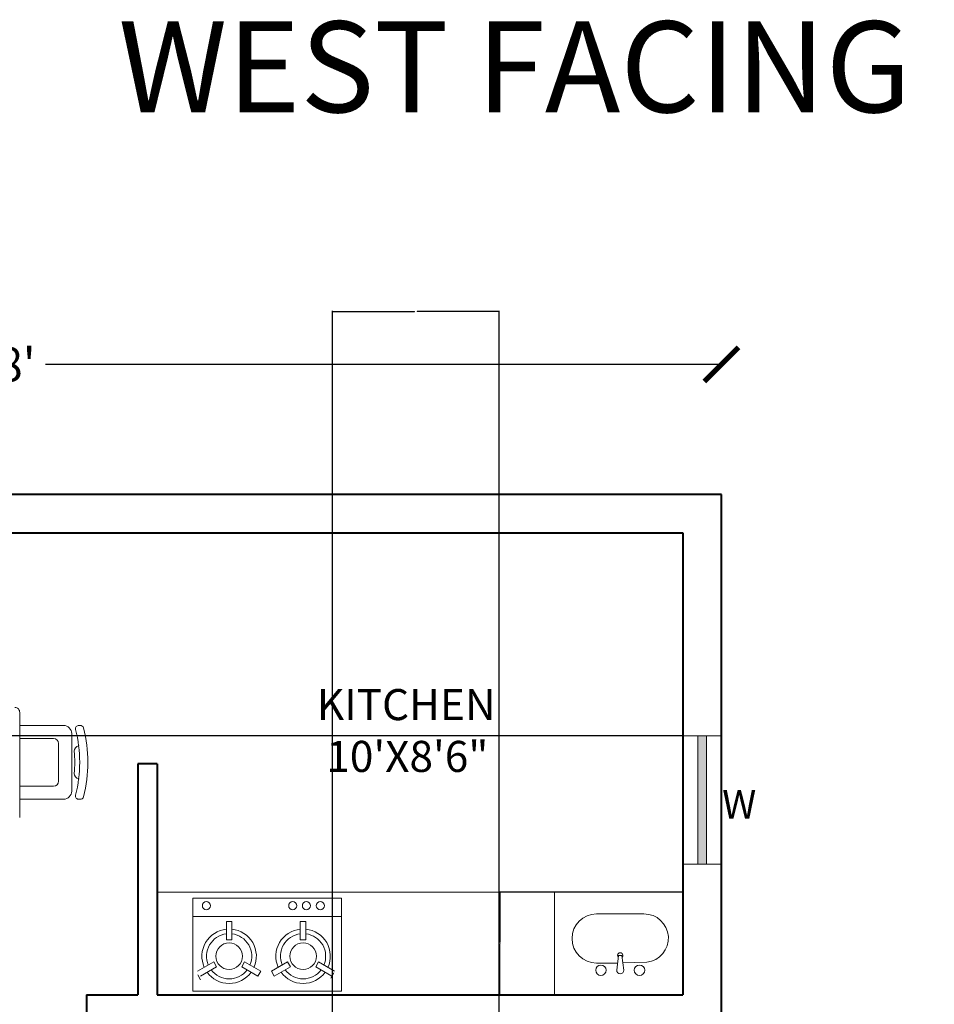
# Model space of a CAD drawing. Units: inches. Extents: x 182 to 1022, y -617 to 111.
# Tile 22 of 33: x 401 to 615, y -120 to 111. Entities that reach past the tile are written whole.
import ezdxf

# ---------------------------------------------------------------- set-up
doc = ezdxf.new("R2010")
doc.units = ezdxf.units.IN
doc.header["$MEASUREMENT"] = 0
for name, color, linetype, lineweight in [('A-ANNO-DIMS', 2, 'Continuous', 18), ('A-ANNO-IDEN', 1, 'Continuous', 18), ('A-ANNO-TEXT', 8, 'Continuous', 20), ('A-AREA-IDEN', 8, 'Continuous', 18), ('A-EQPM', 50, 'Continuous', 18), ('A-FLOR-CASE', 1, 'Continuous', 20), ('A-FLOR-FIXT', 50, 'Continuous', 18), ('A-GLAZ-PATT', 5, 'Continuous', 13), ('wall', 1, 'Continuous', 40), ('wind', 5, 'Continuous', 20)]:
    doc.layers.add(name, color=color, linetype=linetype, lineweight=lineweight)
doc.layers.add('furniture', color=50, linetype='Continuous', lineweight=15, transparency=0.8)
doc.styles.get("Standard").update_dxf_attribs({"font": 'arial.ttf'})
doc.dimstyles.get("Standard").update_dxf_attribs({"dimtxt": 0.18, "dimasz": 0.18, "dimexe": 0.18, "dimexo": 0.0625, "dimgap": 0.09, "dimtad": 0, "dimtih": 1, "dimtoh": 1, "dimdec": 1, "dimzin": 0, "dimdsep": 46, "dimlunit": 4, "dimtxsty": 'Standard', "dimcen": 0.09, "dimadec": 0, "dimazin": 0, "dimtfac": 1, "dimtdec": 1, "dimtofl": 0, "dimtmove": 0, "dimatfit": 3, "dimfxl": 1, "dimtolj": 1, "dimtzin": 0, "dimarcsym": 0})

# ---------------------------------------------------------------- blocks, each defined once
blk = doc.blocks.new('_ArchTick')
at = {"color": 0, "linetype": 'ByBlock', "const_width": 0.15}
blk.add_lwpolyline([(-0.5, -0.5), (0.5, 0.5)], dxfattribs=at)
blk = doc.blocks.new('*D5')
at = {"layer": 'A-ANNO-DIMS', "color": 0, "lineweight": -2, "transparency": 16777216}
for p, q in [((229.36, 30.06), (387.5, 30.06)), ((565.36, 30.06), (407.22, 30.06))]:
    blk.add_line(p, q, dxfattribs=at)
at = {"layer": 'Defpoints', "color": 0, "transparency": 16777216}
for p in [(565.36, 30.06), (229.36, -0.37), (565.36, -0.37)]:
    blk.add_point(p, dxfattribs=at)
at = {"layer": 'A-ANNO-DIMS', "color": 0, "lineweight": -2, "transparency": 16777216, "xscale": 8, "yscale": 8, "zscale": 8, "rotation": 180}
blk.add_blockref('_ArchTick', (229.36, 30.06), dxfattribs=at)
at = {"layer": 'A-ANNO-DIMS', "color": 0, "lineweight": -2, "transparency": 16777216, "xscale": 8, "yscale": 8, "zscale": 8}
blk.add_blockref('_ArchTick', (565.36, 30.06), dxfattribs=at)
at = {"layer": 'A-ANNO-DIMS', "color": 0, "transparency": 16777216, "insert": (397.36, 30.06), "char_height": 8, "attachment_point": 5}
blk.add_mtext("\\A1;28'", dxfattribs=at)
blk = doc.blocks.new('DINING-CHAIR-END')
for p, q in [((5.53, 17.27), (5.92, 17.27)), ((5.7, 17.27), (15.95, 17.27)), ((3.78, 1.92), (3.78, 15.35)), ((8.01, 14.2), (15.95, 14.2)), ((2.16, 12.47), (2.04, 12.47)), ((6.85, 4.22), (6.85, 13.05)), ((2.16, 4.8), (2.04, 4.8)), ((15.95, 3.07), (8.01, 3.07)), ((5.92, 0), (5.53, 0)), ((15.95, 0), (5.7, 0))]:
    blk.add_line(p, q)
for centre, radius, start, end in [((32.95, 8.63), 32.96, 165.853, 194.147), ((1.74, 16.5), 0.768, 84.0784, 165.853), ((1.94, 18.41), 1.15, 264.0784, 275.9216), ((32.95, 8.63), 31.04, 165.6786, 194.3214), ((2.14, 16.5), 0.768, 345.6786, 95.9216), ((5.7, 15.35), 1.92, 90, 180), ((8.01, 13.05), 1.15, 90, 180), ((2.04, 11.32), 1.15, 355.0346, 83.9719), ((32.95, 8.63), 29.89, 175.0346, 184.9654), ((2.04, 5.95), 1.15, 276.0281, 4.9654), ((8.01, 4.22), 1.15, 180, 270), ((1.74, 0.77), 0.768, 194.147, 275.9216), ((1.94, -1.14), 1.15, 84.0784, 95.9216), ((2.14, 0.77), 0.768, 264.0784, 14.3214), ((5.7, 1.92), 1.92, 180, 270)]:
    blk.add_arc(centre, radius, start, end)
blk = doc.blocks.new('*D43')
at = {"layer": 'A-ANNO-DIMS', "color": 0, "lineweight": -2, "transparency": 16777216}
for p, q in [((556.3, -9.37), (186.38, -9.37)), ((186.56, -9.55), (186.56, -32.91)), ((186.56, -56.63), (186.56, -33.28)), ((556.3, -56.81), (186.38, -56.81))]:
    blk.add_line(p, q, dxfattribs=at)
at = {"layer": 'A-ANNO-DIMS', "color": 0, "transparency": 16777216}
for points in [[(186.53, -9.55), (186.59, -9.55), (186.56, -9.37)], [(186.53, -56.63), (186.59, -56.63), (186.56, -56.81)]]:
    blk.add_solid(points, dxfattribs=at)
at = {"layer": 'Defpoints', "color": 0, "transparency": 16777216}
for p in [(556.36, -9.37), (186.56, -56.81), (556.36, -56.81)]:
    blk.add_point(p, dxfattribs=at)
at = {"layer": 'A-ANNO-DIMS', "color": 0, "transparency": 16777216, "insert": (186.56, -33.09), "char_height": 0.18, "attachment_point": 5}
blk.add_mtext('\\A1;3\'-11 1/2"', dxfattribs=at)
blk = doc.blocks.new('*D44')
at = {"layer": 'A-ANNO-DIMS', "color": 0, "lineweight": -2, "transparency": 16777216}
for p, q in [((556.3, -93.37), (513.38, -93.37)), ((513.56, -93.55), (513.56, -105.19)), ((513.56, -117.19), (513.56, -105.56)), ((556.3, -117.37), (513.38, -117.37))]:
    blk.add_line(p, q, dxfattribs=at)
at = {"layer": 'A-ANNO-DIMS', "color": 0, "transparency": 16777216}
for points in [[(513.53, -93.55), (513.59, -93.55), (513.56, -93.37)], [(513.53, -117.19), (513.59, -117.19), (513.56, -117.37)]]:
    blk.add_solid(points, dxfattribs=at)
at = {"layer": 'Defpoints', "color": 0, "transparency": 16777216}
for p in [(513.56, -93.37), (556.36, -93.37), (556.36, -117.37)]:
    blk.add_point(p, dxfattribs=at)
at = {"layer": 'A-ANNO-DIMS', "color": 0, "transparency": 16777216, "insert": (513.56, -105.37), "char_height": 0.18, "attachment_point": 5}
blk.add_mtext('\\A1;2\'-0"', dxfattribs=at)
blk = doc.blocks.new('*D47')
at = {"layer": 'A-ANNO-DIMS', "color": 0, "lineweight": -2, "transparency": 16777216}
for p, q in [((474.36, -396.31), (474.36, 42.61)), ((474.54, 42.43), (493.53, 42.43)), ((513.18, 42.43), (494.19, 42.43)), ((513.36, -400.31), (513.36, 42.61))]:
    blk.add_line(p, q, dxfattribs=at)
at = {"layer": 'A-ANNO-DIMS', "color": 0, "transparency": 16777216}
for points in [[(474.54, 42.46), (474.54, 42.4), (474.36, 42.43)], [(513.18, 42.46), (513.18, 42.4), (513.36, 42.43)]]:
    blk.add_solid(points, dxfattribs=at)
at = {"layer": 'Defpoints', "color": 0, "transparency": 16777216}
for p in [(513.36, 42.43), (474.36, -396.37), (513.36, -400.37)]:
    blk.add_point(p, dxfattribs=at)
at = {"layer": 'A-ANNO-DIMS', "color": 0, "transparency": 16777216, "insert": (493.86, 42.43), "char_height": 0.18, "attachment_point": 5}
blk.add_mtext('\\A1;3\'-3"', dxfattribs=at)

msp = doc.modelspace()

# ---------------------------------------------------------------- hatches: boundary and pattern name
at = {"layer": 'A-GLAZ-PATT'}
h = msp.add_hatch(color=256, dxfattribs=at)
h.dxf.hatch_style = 1
h.paths.add_polyline_path([(285.4, -3.87), (255.4, -3.87), (255.4, -5.87), (285.4, -5.87)])
h.paths.add_polyline_path([(376.09, -3.87), (340.09, -3.87), (340.09, -5.87), (376.09, -5.87)])
h.paths.add_polyline_path([(561.86, -132.92), (559.86, -132.92), (559.86, -168.92), (561.86, -168.92)])
h.paths.add_polyline_path([(561.86, -56.81), (559.86, -56.81), (559.86, -86.81), (561.86, -86.81)])
h.paths.add_polyline_path([(561.86, -258.37), (559.86, -258.37), (559.86, -282.37), (561.86, -282.37)])
h.paths.add_polyline_path([(533.36, -534.87), (497.36, -534.87), (497.36, -536.87), (533.36, -536.87)])
h.paths.add_polyline_path([(234.86, -252.37), (232.86, -252.37), (232.86, -288.37), (234.86, -288.37)])

# ---------------------------------------------------------------- linework, layer by layer
at = {"layer": 'A-EQPM'}
for p, q in [((441.69, -94.77), (476.49, -94.77)), ((441.69, -94.77), (441.69, -116.52)), ((476.49, -94.77), (476.49, -116.52)), ((441.69, -99.12), (476.49, -99.12)), ((449.55, -104.57), (449.55, -100.24)), ((449.55, -100.24), (450.86, -100.24)), ((450.86, -104.57), (450.86, -100.24)), ((466.85, -104.57), (466.85, -100.24)), ((466.85, -100.24), (468.15, -100.24)), ((468.15, -104.57), (468.15, -100.24)), ((449.55, -104.57), (450.86, -104.57)), ((466.85, -104.57), (468.15, -104.57)), ((446.58, -109.72), (442.82, -111.88)), ((447.23, -110.85), (446.58, -109.72)), ((453.83, -109.72), (453.17, -110.85)), ((453.83, -109.72), (457.58, -111.89)), ((463.87, -109.72), (460.12, -111.88)), ((464.52, -110.85), (463.87, -109.72)), ((471.12, -109.72), (470.47, -110.85)), ((471.12, -109.72), (474.87, -111.89)), ((443.5, -113.87), (442.85, -112.74)), ((447.23, -110.85), (443.48, -113.02)), ((453.17, -110.85), (456.93, -113.02)), ((457.58, -111.89), (456.93, -113.02)), ((460.77, -113.02), (460.12, -111.88)), ((464.52, -110.85), (460.77, -113.02)), ((470.47, -110.85), (474.22, -113.02)), ((474.72, -112.24), (474, -113.49)), ((441.69, -116.52), (476.49, -116.52))]:
    msp.add_line(p, q, dxfattribs=at)
at = {"layer": 'A-EQPM', "extrusion": (0, 0, -1)}
for centre, major_axis, start_param, end_param in [((444.87, -96.55), (0.667, -0.667), 2.35619449019219, 8.639379797371777), ((465.07, -96.55), (0.667, -0.667), 2.35619449019219, 8.639379797371777), ((468.27, -96.55), (0.667, -0.667), 2.35619449019219, 8.639379797371777), ((471.54, -96.55), (0.667, -0.667), 2.35619449019219, 8.639379797371777), ((450.2, -108.38), (-0.01, -6.37), 1.14879, 3.038067), ((450.2, -108.38), (-3.74, -3.74), 0.385932, 2.23281), ((450.2, -108.38), (0, -6.37), 3.244173, 5.13345), ((450.2, -108.38), (-3.74, -3.74), 2.480327, 4.327205), ((467.5, -108.38), (-0.01, -6.37), 1.148752, 3.038029), ((467.5, -108.38), (-3.74, -3.74), 0.385932, 2.23281), ((467.5, -108.38), (0, -6.37), 3.2451, 5.134376), ((467.5, -108.38), (3.74, -3.74), 4.051123, 5.898002), ((450.2, -108.38), (2.2, -2.2), 2.356194490192306, 8.639379797371893), ((467.5, -108.38), (2.2, -2.2), 2.356194490192312, 8.639379797371898), ((450.2, -108.38), (0, -6.37), -0.944011, 0.945266), ((450.2, -108.38), (3.74, -3.74), 6.145519, 7.992397), ((467.5, -108.38), (0.01, -6.37), -0.942584, 0.946692), ((467.5, -108.38), (3.74, -3.74), 6.145519, 7.992397)]:
    msp.add_ellipse(centre, major_axis=major_axis, ratio=1, start_param=start_param, end_param=end_param, dxfattribs=at)
at = {"layer": 'A-FLOR-CASE'}
for p, q in [((433.36, -93.37), (556.36, -93.37)), ((526.31, -93.37), (526.31, -117.37))]:
    msp.add_line(p, q, dxfattribs=at)
at = {"layer": 'A-FLOR-FIXT'}
for p, q in [((547.23, -98.49), (536.17, -98.49)), ((540.88, -111.66), (541.29, -108.18)), ((541.23, -108.18), (542.11, -108.18)), ((542.11, -108.18), (542.52, -111.66)), ((541.08, -109.97), (536.17, -109.97)), ((547.95, -109.76), (542.31, -109.92))]:
    msp.add_line(p, q, dxfattribs=at)
for centre in [(537.19, -111.66), (546.21, -111.66)]:
    msp.add_circle(centre, 1.23, dxfattribs=at)
for centre, radius, start, end in [((536.17, -104.23), 5.74, 90, 270), ((547.32, -104.14), 5.65, 276.3659, 90.8792), ((541.7, -108.18), 0.615, 318.1701, 221.8299), ((541.7, -111.66), 0.82, 180, 0)]:
    msp.add_arc(centre, radius, start, end, dxfattribs=at)
at = {"layer": 'furniture'}
msp.add_line((401.19, -75.91), (401.19, -51.35), dxfattribs=at)
msp.add_arc((400.1, -51.3), 1.1, 357.166, 92.834, dxfattribs=at)
at = {"layer": 'wall'}
for p, q in [((565.36, -0.37), (229.36, -0.37)), ((565.36, -540.37), (565.36, -0.37)), ((238.36, -9.37), (556.36, -9.37)), ((556.36, -9.37), (556.36, -117.37)), ((428.86, -63.37), (428.86, -117.37)), ((433.36, -63.37), (428.86, -63.37)), ((433.36, -63.37), (433.36, -117.37)), ((416.86, -117.37), (428.86, -117.37)), ((416.86, -117.37), (416.86, -121.87)), ((433.36, -117.37), (556.36, -117.37))]:
    msp.add_line(p, q, dxfattribs=at)
at = {"layer": 'wind'}
for p, q in [((556.36, -56.81), (565.36, -56.81)), ((559.86, -56.81), (559.86, -86.81)), ((561.86, -56.81), (561.86, -86.81)), ((556.36, -86.81), (565.36, -86.81))]:
    msp.add_line(p, q, dxfattribs=at)

# ---------------------------------------------------------------- block references
at = {"layer": 'furniture', "rotation": 180}
msp.add_blockref('DINING-CHAIR-END', (417.14, -54.39), dxfattribs=at)

# ---------------------------------------------------------------- texts
at = {"layer": 'A-ANNO-IDEN'}
msp.add_text('W', height=6.65, dxfattribs=at).set_placement((565.56, -76.17))
at = {"layer": 'A-ANNO-TEXT', "insert": (424.27, 110.32), "char_height": 21.2807, "attachment_point": 1}
msp.add_mtext_dynamic_manual_height_columns('WEST FACING HOUSE', width=345.7385, gutter_width=3.55, heights=[0], dxfattribs=at)
at = {"layer": 'A-AREA-IDEN', "insert": (461.83, -45.88), "char_height": 7.2703, "attachment_point": 1}
msp.add_mtext_dynamic_manual_height_columns('    KITCHEN\\P     10\'X8\'6"', width=65.8887, gutter_width=1.21, heights=[0], dxfattribs=at)

# ---------------------------------------------------------------- dimensions: what is measured, and where the dimension line sits
at = {"layer": 'A-ANNO-DIMS'}
for base, p1, p2, override, picture, middle in [((513.36, 42.43), (474.36, -396.37), (513.36, -400.37), {"dimdec": 1, "dimlfac": 1, "dimrnd": 0, "dimzin": 1, "dimdsep": 46, "dimlunit": 4, "dimfrac": 2}, '*D47', (493.86, 42.43)), ((565.36, 30.06), (229.36, -0.37), (565.36, -0.37), {"dimtxt": 8, "dimasz": 8, "dimgap": 3, "dimblk1": 'ArchTick', "dimblk2": 'ArchTick', "dimsah": 1, "dimse1": 1, "dimse2": 1, "dimsd1": 0, "dimclrd": 0, "dimclre": 0, "dimclrt": 0}, '*D5', (397.36, 30.06))]:
    dim = msp.add_linear_dim(base=base, p1=p1, p2=p2, dimstyle='Standard', override=override, dxfattribs=at)
    dim.commit()
    dim.dimension.update_dxf_attribs({"geometry": picture, "text_midpoint": middle})
for base, p1, p2, picture, middle in [((186.56, -56.81), (556.36, -9.37), (556.36, -56.81), '*D43', (186.56, -33.09)), ((513.56, -93.37), (556.36, -117.37), (556.36, -93.37), '*D44', (513.56, -105.37))]:
    dim = msp.add_linear_dim(base=base, p1=p1, p2=p2, angle=90, dimstyle='Standard', override={"dimdec": 1, "dimlfac": 1, "dimrnd": 0, "dimzin": 1, "dimdsep": 46, "dimlunit": 4, "dimfrac": 2}, dxfattribs=at)
    dim.commit()
    dim.dimension.update_dxf_attribs({"geometry": picture, "text_midpoint": middle})

doc.saveas('drawing.dxf')
